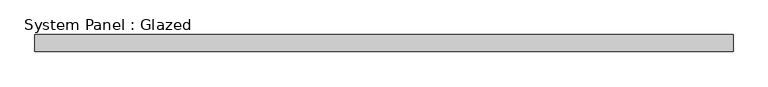
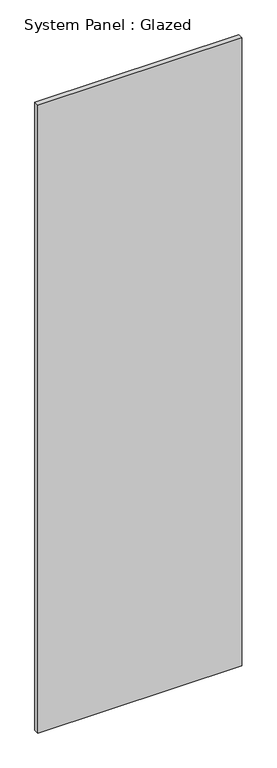
"""IFC4 building model written with IfcOpenShell, lengths in millimetres: plate geometry, System Panel : Glazed."""

from ifc_helpers import new_model, si_unit, origin, origin_with_axes, place, context, project, spatial, polyline, outline, extrude, source, transform, mapped, element, save


def system_panel_glazed_0d5058d0(model_context):
    return source(origin(), model_context, "Body", "SweptSolid", [
        extrude(outline(polyline([(519.45, 19.05), (-519.45, 19.05), (-519.45, 44.45), (519.45, 44.45), (519.45, 19.05)])), origin_with_axes(), (0.0, 0.0, 1.0), 3379.9820397),
    ])


if __name__ == "__main__":
    model = new_model("IFC4")
    model_context = context("Model", 3, world=origin())
    ifc_project = project(units=[si_unit("LENGTHUNIT", "METRE", prefix="MILLI")], contexts=[model_context])
    site = spatial("IfcSite", under=ifc_project)
    building = spatial("IfcBuilding", under=site)
    placement = place(None, origin())
    system_panel_glazed_shape = system_panel_glazed_0d5058d0(model_context)
    element("IfcPlate", 1, ObjectType="System Panel : Glazed", at=placement, inside=building, context=model_context, shape_type="MappedRepresentation", body=[
        mapped(system_panel_glazed_shape, transform((0.0, 0.0, 0.0), x_axis=(1.0, 0.0, 0.0), y_axis=(0.0, 1.0, 0.0), z_axis=(0.0, 0.0, 1.0))),
    ])
    save(model, "model.ifc")

# Revit data of these elements
# Type "System Panel : Glazed"
#   Construction Type Id = "GSP4R"
#   Analytic Construction = "1/8 in Pilkington single glazing"
#   Visual Light Transmittance = 0.9
#   Solar Heat Gain Coefficient = 0.86
#   Heat Transfer Coefficient (U) = 1.18115 BTU/(h·ft²·°F)
#   Define Thermal Properties by = 1
# Element 1 (IfcPlate, "System Panel : Glazed")
#   Materials on its faces: "Glass"
# Materials
#   "Glass": class "Glass", colour RGB 0 128 192, transparency 0.75, Description = "Soda Lime Glass", Cost = 0
